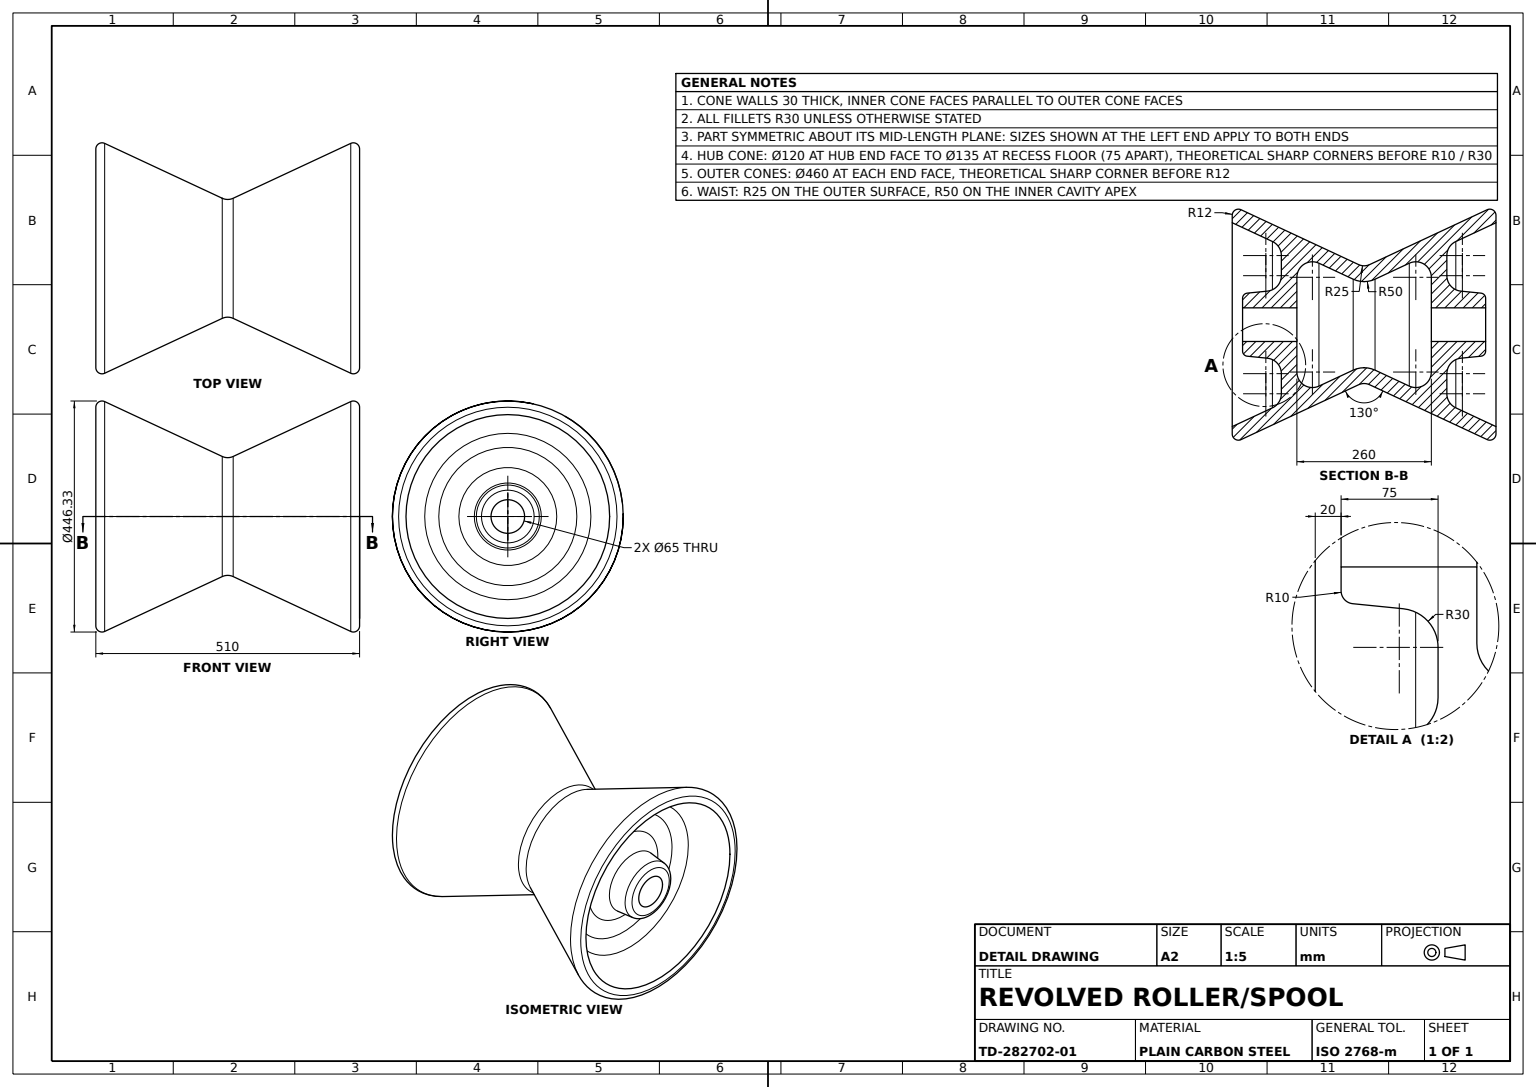
from build123d import *


with BuildPart() as part:
    # Pulley Profile Sketch → Pulley Body Revolve (revolve)
    with BuildSketch(Plane.XY, mode=Mode.PRIVATE) as pulley_body_revolve_sk:
        with BuildLine():
            Line((130, 32.5), (235, 32.5))
            Line((235, 32.5), (235, 50.950124379))
            ThreePointArc((235, 50.950124379), (232.414525336, 57.660177586), (225.99503719, 60.900496281))
            Line((225.99503719, 60.900496281), (187.014888429, 64.798511157))
            ThreePointArc((187.014888429, 64.798511157), (167.756423993, 74.519467241), (160, 94.649626863))
            Line((160, 94.649626863), (160, 133.487327082))
            ThreePointArc((160, 133.487327082), (164.698256626, 149.606315333), (177.321452148, 160.676560693))
            Line((177.321452148, 160.676560693), (255, 196.898662431))
            Line((255, 196.898662431), (255, 211.163773075))
            ThreePointArc((255, 211.163773075), (249.4475953, 221.284470424), (237.928580859, 222.039466519))
            Line((237.928580859, 222.039466519), (10.565456544, 116.018300469))
            ThreePointArc((10.565456544, 116.018300469), (0, 113.675995145), (-10.565456544, 116.018300469))
            Line((-10.565456544, 116.018300469), (-237.928580859, 222.039466519))
            ThreePointArc((-237.928580859, 222.039466519), (-249.4475953, 221.284470424), (-255, 211.163773075))
            Line((-255, 211.163773075), (-255, 196.898662431))
            Line((-255, 196.898662431), (-177.321452148, 160.676560693))
            ThreePointArc((-177.321452148, 160.676560693), (-164.698256626, 149.606315333), (-160, 133.487327082))
            Line((-160, 133.487327082), (-160, 94.649626863))
            ThreePointArc((-160, 94.649626863), (-167.756423993, 74.519467241), (-187.014888429, 64.798511157))
            Line((-187.014888429, 64.798511157), (-225.99503719, 60.900496281))
            ThreePointArc((-225.99503719, 60.900496281), (-232.414525336, 57.660177586), (-235, 50.950124379))
            Line((-235, 50.950124379), (-235, 32.5))
            Line((-235, 32.5), (-130, 32.5))
            Line((-130, 32.5), (-130, 91.519637848))
            ThreePointArc((-130, 91.519637848), (-116.11898825, 116.821381223), (-87.321452148, 118.708871459))
            Line((-87.321452148, 118.708871459), (-21.130913087, 87.843716198))
            ThreePointArc((-21.130913087, 87.843716198), (0, 83.15910555), (21.130913087, 87.843716198))
            Line((21.130913087, 87.843716198), (87.321452148, 118.708871459))
            ThreePointArc((87.321452148, 118.708871459), (116.11898825, 116.821381223), (130, 91.519637848))
            Line((130, 91.519637848), (130, 32.5))
        make_face()
    revolve(pulley_body_revolve_sk.sketch.rotate(Axis((0, 0, 0), (1, 0, 0)), 90), axis=Axis((0, 0, 0), (1, 0, 0)))


solid = part.part
